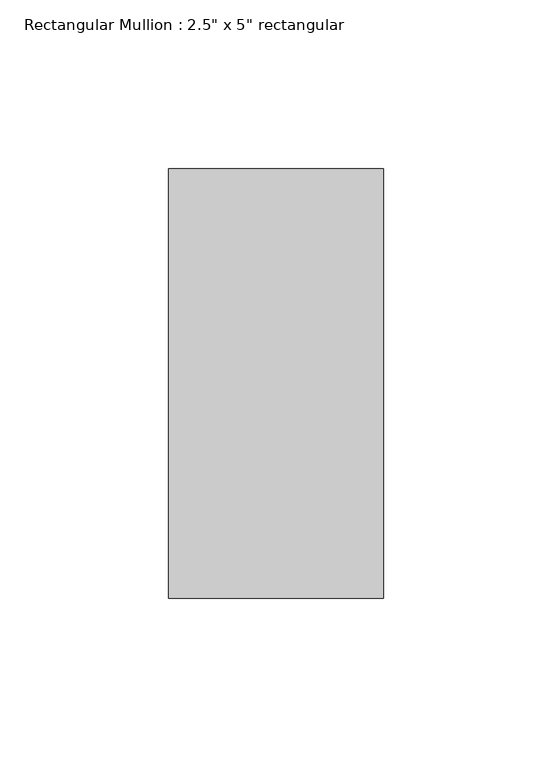
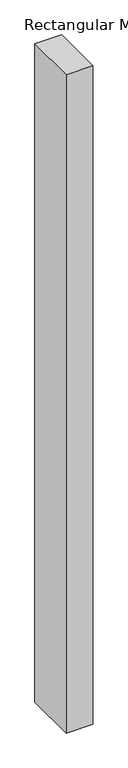
"""IFC4 building model written with IfcOpenShell, lengths in millimetres: member geometry."""

from ifc_helpers import new_model, si_unit, frame, origin, place, context, project, spatial, polyline, outline, extrude, source, transform, mapped, element, save


def member_dc22f6be(model_context):
    return source(origin(), model_context, "Body", "SweptSolid", [
        extrude(outline(polyline([(0.0, 63.5), (0.0, -63.5), (-63.5, -63.5), (-63.5, 63.5), (0.0, 63.5)])), frame((0.0, 0.0, -1639.8191133), z_axis=(0.0, 0.0, 1.0), x_axis=(1.0, 0.0, 0.0)), (0.0, 0.0, 1.0), 1639.8191133),
    ])


if __name__ == "__main__":
    model = new_model("IFC4")
    model_context = context("Model", 3, world=origin())
    ifc_project = project(units=[si_unit("LENGTHUNIT", "METRE", prefix="MILLI")], contexts=[model_context])
    site = spatial("IfcSite", under=ifc_project)
    building = spatial("IfcBuilding", under=site)
    placement = place(None, origin())
    member_shape = member_dc22f6be(model_context)
    element("IfcMember", 1, ObjectType="Rectangular Mullion : 2.5\" x 5\" rectangular", at=placement, inside=building, context=model_context, shape_type="MappedRepresentation", body=[
        mapped(member_shape, transform((0.0, 0.0, 0.0), x_axis=(1.0, 0.0, 0.0), y_axis=(0.0, 1.0, 0.0), z_axis=(0.0, 0.0, 1.0))),
    ])
    save(model, "model.ifc")

# Revit data of these elements
# Type "Rectangular Mullion : 2.5\" x 5\" rectangular"
#   built-in parameter 1007304 = 0.416667 (stored number, unit not read)
#   built-in parameter 1007301 = 0.104167 (stored number, unit not read)
#   built-in parameter 1007300 = 0.104167 (stored number, unit not read)
# Element 1 (IfcMember, "Rectangular Mullion : 2.5\" x 5\" rectangular")
#   Materials on its faces: "Aluminum"
# Materials
#   "Aluminum": class "Metal", colour RGB 247 247 247, transparency 0, Description = "Aluminum 6061", Cost = 0
